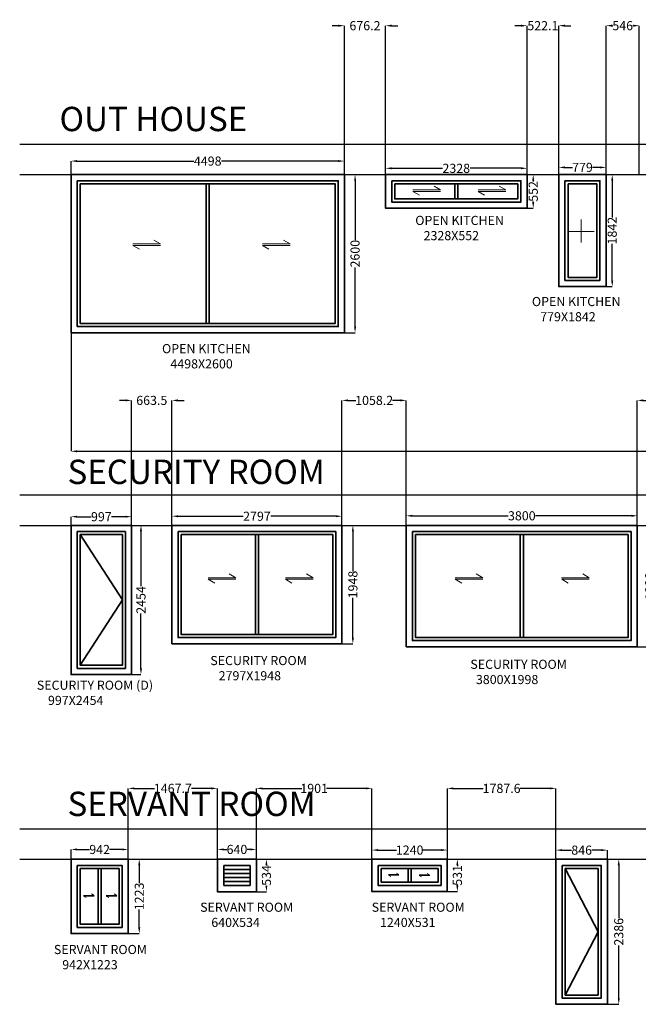
# Model space of a CAD drawing. Units: millimetres. Extents: x 16338 to 57165, y -4429 to 26237.
# Tile 4 of 6: x 18335 to 28512, y 10044 to 26237. Entities that reach past the tile are written whole.
import ezdxf

# ---------------------------------------------------------------- set-up
doc = ezdxf.new("R2010")
doc.units = ezdxf.units.MM
doc.header["$MEASUREMENT"] = 0
for name, color, linetype, lineweight in [('A-ANNO-DIMS', 5, 'Continuous', 18), ('A-ANNO-SYMB', 4, 'Continuous', 18), ('A-ANNO-TEXT', 3, 'Continuous', 18), ('A-ELEV', 8, 'Continuous', 25), ('A-GLAZ', 7, 'Continuous', 35)]:
    doc.layers.add(name, color=color, linetype=linetype, lineweight=lineweight)
doc.styles.get("Standard").update_dxf_attribs({"font": 'arial.ttf'})
doc.dimstyles.get("Standard").update_dxf_attribs({"dimtxt": 150, "dimasz": 100, "dimexe": 0.18, "dimexo": 0.0625, "dimgap": 0.09, "dimtad": 0, "dimdec": 0, "dimzin": 0, "dimdsep": 46, "dimtxsty": 'Standard', "dimcen": 0.09, "dimadec": 0, "dimazin": 0, "dimtfac": 1, "dimtdec": 0, "dimtofl": 0, "dimtmove": 0, "dimatfit": 3, "dimfxl": 1, "dimtolj": 1, "dimtzin": 0, "dimarcsym": 0})

# ---------------------------------------------------------------- blocks, each defined once
blk = doc.blocks.new('*D1')
at = {"layer": 'A-ANNO-DIMS', "color": 0, "lineweight": -2, "transparency": 16777216}
for p, q in [((23677, 23689), (23853, 23689)), ((23852, 23589), (23852, 22614)), ((23852, 21189), (23852, 22164)), ((23677, 21089), (23853, 21089))]:
    blk.add_line(p, q, dxfattribs=at)
at = {"layer": 'A-ANNO-DIMS', "color": 0, "transparency": 16777216}
for points in [[(23836, 23589), (23869, 23589), (23852, 23689)], [(23836, 21189), (23869, 21189), (23852, 21089)]]:
    blk.add_solid(points, dxfattribs=at)
at = {"layer": 'Defpoints', "color": 0, "transparency": 16777216}
for p in [(23677, 23689), (23677, 21089), (23852, 21089)]:
    blk.add_point(p, dxfattribs=at)
at = {"layer": 'A-ANNO-DIMS', "color": 0, "transparency": 16777216, "insert": (23852, 22389), "char_height": 150, "attachment_point": 5, "rotation": 90}
blk.add_mtext('\\A1;2600', dxfattribs=at)
blk = doc.blocks.new('*D2')
at = {"layer": 'A-ANNO-DIMS', "color": 0, "lineweight": -2, "transparency": 16777216}
for p, q in [((24353, 23689), (24353, 23793)), ((24453, 23793), (25292, 23793)), ((26581, 23793), (25743, 23793)), ((26681, 23689), (26681, 23793))]:
    blk.add_line(p, q, dxfattribs=at)
at = {"layer": 'A-ANNO-DIMS', "color": 0, "transparency": 16777216}
for points in [[(24453, 23810), (24453, 23777), (24353, 23793)], [(26581, 23810), (26581, 23777), (26681, 23793)]]:
    blk.add_solid(points, dxfattribs=at)
at = {"layer": 'Defpoints', "color": 0, "transparency": 16777216}
for p in [(24353, 23689), (26681, 23793), (26681, 23689)]:
    blk.add_point(p, dxfattribs=at)
at = {"layer": 'A-ANNO-DIMS', "color": 0, "transparency": 16777216, "insert": (25517, 23793), "char_height": 150, "attachment_point": 5}
blk.add_mtext('\\A1;2328', dxfattribs=at)
blk = doc.blocks.new('*D3')
at = {"layer": 'A-ANNO-DIMS', "color": 0, "lineweight": -2, "transparency": 16777216}
for p, q in [((26681, 23689), (26783, 23689)), ((26783, 23589), (26783, 23578)), ((26783, 23237), (26783, 23248)), ((26681, 23137), (26783, 23137))]:
    blk.add_line(p, q, dxfattribs=at)
at = {"layer": 'A-ANNO-DIMS', "color": 0, "transparency": 16777216}
for points in [[(26766, 23589), (26799, 23589), (26783, 23689)], [(26766, 23237), (26799, 23237), (26783, 23137)]]:
    blk.add_solid(points, dxfattribs=at)
at = {"layer": 'Defpoints', "color": 0, "transparency": 16777216}
for p in [(26681, 23689), (26681, 23137), (26783, 23137)]:
    blk.add_point(p, dxfattribs=at)
at = {"layer": 'A-ANNO-DIMS', "color": 0, "transparency": 16777216, "insert": (26783, 23413), "char_height": 150, "attachment_point": 5, "rotation": 90}
blk.add_mtext('\\A1;552', dxfattribs=at)
blk = doc.blocks.new('*D4')
at = {"layer": 'A-ANNO-DIMS', "color": 0, "lineweight": -2, "transparency": 16777216}
for p, q in [((27203, 23689), (27203, 23808)), ((27303, 23808), (27428, 23808)), ((27882, 23808), (27758, 23808)), ((27982, 23689), (27982, 23808))]:
    blk.add_line(p, q, dxfattribs=at)
at = {"layer": 'A-ANNO-DIMS', "color": 0, "transparency": 16777216}
for points in [[(27303, 23824), (27303, 23791), (27203, 23808)], [(27882, 23824), (27882, 23791), (27982, 23808)]]:
    blk.add_solid(points, dxfattribs=at)
at = {"layer": 'Defpoints', "color": 0, "transparency": 16777216}
for p in [(27982, 23808), (27203, 23689), (27982, 23689)]:
    blk.add_point(p, dxfattribs=at)
at = {"layer": 'A-ANNO-DIMS', "color": 0, "transparency": 16777216, "insert": (27593, 23808), "char_height": 150, "attachment_point": 5}
blk.add_mtext('\\A1;779', dxfattribs=at)
blk = doc.blocks.new('*D5')
at = {"layer": 'A-ANNO-DIMS', "color": 0, "lineweight": -2, "transparency": 16777216}
for p, q in [((27982, 23689), (28083, 23689)), ((28082, 23589), (28082, 22984)), ((28082, 21947), (28082, 22552)), ((27982, 21847), (28083, 21847))]:
    blk.add_line(p, q, dxfattribs=at)
at = {"layer": 'A-ANNO-DIMS', "color": 0, "transparency": 16777216}
for points in [[(28066, 23589), (28099, 23589), (28082, 23689)], [(28066, 21947), (28099, 21947), (28082, 21847)]]:
    blk.add_solid(points, dxfattribs=at)
at = {"layer": 'Defpoints', "color": 0, "transparency": 16777216}
for p in [(27982, 23689), (27982, 21847), (28082, 21847)]:
    blk.add_point(p, dxfattribs=at)
at = {"layer": 'A-ANNO-DIMS', "color": 0, "transparency": 16777216, "insert": (28082, 22768), "char_height": 150, "attachment_point": 5, "rotation": 90}
blk.add_mtext('\\A1;1842', dxfattribs=at)
blk = doc.blocks.new('*D20')
at = {"layer": 'A-ANNO-DIMS', "color": 0, "lineweight": -2, "transparency": 16777216}
for p, q in [((19179, 17921), (19179, 18063)), ((19279, 18063), (19512, 18063)), ((20076, 18063), (19843, 18063)), ((20176, 17921), (20176, 18063))]:
    blk.add_line(p, q, dxfattribs=at)
at = {"layer": 'A-ANNO-DIMS', "color": 0, "transparency": 16777216}
for points in [[(19279, 18080), (19279, 18047), (19179, 18063)], [(20076, 18080), (20076, 18047), (20176, 18063)]]:
    blk.add_solid(points, dxfattribs=at)
at = {"layer": 'Defpoints', "color": 0, "transparency": 16777216}
for p in [(20176, 18063), (19179, 17921), (20176, 17921)]:
    blk.add_point(p, dxfattribs=at)
at = {"layer": 'A-ANNO-DIMS', "color": 0, "transparency": 16777216, "insert": (19678, 18063), "char_height": 150, "attachment_point": 5}
blk.add_mtext('\\A1;997', dxfattribs=at)
blk = doc.blocks.new('*D21')
at = {"layer": 'A-ANNO-DIMS', "color": 0, "lineweight": -2, "transparency": 16777216}
for p, q in [((20176, 17921), (20330, 17921)), ((20330, 17821), (20330, 16919)), ((20330, 15567), (20330, 16469)), ((20176, 15467), (20330, 15467))]:
    blk.add_line(p, q, dxfattribs=at)
at = {"layer": 'A-ANNO-DIMS', "color": 0, "transparency": 16777216}
for points in [[(20313, 17821), (20347, 17821), (20330, 17921)], [(20313, 15567), (20347, 15567), (20330, 15467)]]:
    blk.add_solid(points, dxfattribs=at)
at = {"layer": 'Defpoints', "color": 0, "transparency": 16777216}
for p in [(20176, 17921), (20176, 15467), (20330, 15467)]:
    blk.add_point(p, dxfattribs=at)
at = {"layer": 'A-ANNO-DIMS', "color": 0, "transparency": 16777216, "insert": (20330, 16694), "char_height": 150, "attachment_point": 5, "rotation": 90}
blk.add_mtext('\\A1;2454', dxfattribs=at)
blk = doc.blocks.new('*D22')
at = {"layer": 'A-ANNO-DIMS', "color": 0, "lineweight": -2, "transparency": 16777216}
for p, q in [((20840, 17921), (20840, 18071)), ((20940, 18071), (22013, 18071)), ((23537, 18071), (22464, 18071)), ((23637, 17921), (23637, 18071))]:
    blk.add_line(p, q, dxfattribs=at)
at = {"layer": 'A-ANNO-DIMS', "color": 0, "transparency": 16777216}
for points in [[(20940, 18087), (20940, 18054), (20840, 18071)], [(23537, 18087), (23537, 18054), (23637, 18071)]]:
    blk.add_solid(points, dxfattribs=at)
at = {"layer": 'Defpoints', "color": 0, "transparency": 16777216}
for p in [(23637, 18071), (20840, 17921), (23637, 17921)]:
    blk.add_point(p, dxfattribs=at)
at = {"layer": 'A-ANNO-DIMS', "color": 0, "transparency": 16777216, "insert": (22238, 18071), "char_height": 150, "attachment_point": 5}
blk.add_mtext('\\A1;2797', dxfattribs=at)
blk = doc.blocks.new('*D23')
at = {"layer": 'A-ANNO-DIMS', "color": 0, "lineweight": -2, "transparency": 16777216}
for p, q in [((23637, 17921), (23816, 17921)), ((23816, 17821), (23816, 17164)), ((23816, 16073), (23816, 16730)), ((23637, 15973), (23816, 15973))]:
    blk.add_line(p, q, dxfattribs=at)
at = {"layer": 'A-ANNO-DIMS', "color": 0, "transparency": 16777216}
for points in [[(23799, 17821), (23833, 17821), (23816, 17921)], [(23799, 16073), (23833, 16073), (23816, 15973)]]:
    blk.add_solid(points, dxfattribs=at)
at = {"layer": 'Defpoints', "color": 0, "transparency": 16777216}
for p in [(23637, 17921), (23637, 15973), (23816, 15973)]:
    blk.add_point(p, dxfattribs=at)
at = {"layer": 'A-ANNO-DIMS', "color": 0, "transparency": 16777216, "insert": (23816, 16947), "char_height": 150, "attachment_point": 5, "rotation": 90}
blk.add_mtext('\\A1;1948', dxfattribs=at)
blk = doc.blocks.new('*D24')
at = {"layer": 'A-ANNO-DIMS', "color": 0, "lineweight": -2, "transparency": 16777216}
for p, q in [((24695, 17921), (24695, 18078)), ((24795, 18078), (26371, 18078)), ((28395, 18078), (26819, 18078)), ((28495, 17921), (28495, 18078))]:
    blk.add_line(p, q, dxfattribs=at)
at = {"layer": 'A-ANNO-DIMS', "color": 0, "transparency": 16777216}
for points in [[(24795, 18095), (24795, 18061), (24695, 18078)], [(28395, 18095), (28395, 18061), (28495, 18078)]]:
    blk.add_solid(points, dxfattribs=at)
at = {"layer": 'Defpoints', "color": 0, "transparency": 16777216}
for p in [(28495, 18078), (24695, 17921), (28495, 17921)]:
    blk.add_point(p, dxfattribs=at)
at = {"layer": 'A-ANNO-DIMS', "color": 0, "transparency": 16777216, "insert": (26595, 18078), "char_height": 150, "attachment_point": 5}
blk.add_mtext('\\A1;3800', dxfattribs=at)
blk = doc.blocks.new('*D25')
at = {"layer": 'A-ANNO-DIMS', "color": 0, "lineweight": -2, "transparency": 16777216}
for p, q in [((28495, 17921), (28700, 17921)), ((28700, 17821), (28700, 17139)), ((28700, 16023), (28700, 16705)), ((28495, 15923), (28700, 15923))]:
    blk.add_line(p, q, dxfattribs=at)
at = {"layer": 'A-ANNO-DIMS', "color": 0, "transparency": 16777216}
for points in [[(28683, 17821), (28717, 17821), (28700, 17921)], [(28683, 16023), (28717, 16023), (28700, 15923)]]:
    blk.add_solid(points, dxfattribs=at)
at = {"layer": 'Defpoints', "color": 0, "transparency": 16777216}
for p in [(28495, 17921), (28495, 15923), (28700, 15923)]:
    blk.add_point(p, dxfattribs=at)
at = {"layer": 'A-ANNO-DIMS', "color": 0, "transparency": 16777216, "insert": (28700, 16922), "char_height": 150, "attachment_point": 5, "rotation": 90}
blk.add_mtext('\\A1;1998', dxfattribs=at)
blk = doc.blocks.new('*D40')
at = {"layer": 'A-ANNO-DIMS', "color": 0, "lineweight": -2, "transparency": 16777216}
for p, q in [((19179, 12430), (19179, 12591)), ((19279, 12590), (19485, 12590)), ((20021, 12590), (19815, 12590)), ((20121, 12430), (20121, 12591))]:
    blk.add_line(p, q, dxfattribs=at)
at = {"layer": 'A-ANNO-DIMS', "color": 0, "transparency": 16777216}
for points in [[(19279, 12607), (19279, 12574), (19179, 12590)], [(20021, 12607), (20021, 12574), (20121, 12590)]]:
    blk.add_solid(points, dxfattribs=at)
at = {"layer": 'Defpoints', "color": 0, "transparency": 16777216}
for p in [(20121, 12590), (19179, 12430), (20121, 12430)]:
    blk.add_point(p, dxfattribs=at)
at = {"layer": 'A-ANNO-DIMS', "color": 0, "transparency": 16777216, "insert": (19650, 12590), "char_height": 150, "attachment_point": 5}
blk.add_mtext('\\A1;942', dxfattribs=at)
blk = doc.blocks.new('*D41')
at = {"layer": 'A-ANNO-DIMS', "color": 0, "lineweight": -2, "transparency": 16777216}
for p, q in [((20121, 12430), (20302, 12430)), ((20302, 12330), (20302, 12035)), ((20302, 11307), (20302, 11601)), ((20121, 11207), (20302, 11207))]:
    blk.add_line(p, q, dxfattribs=at)
at = {"layer": 'A-ANNO-DIMS', "color": 0, "transparency": 16777216}
for points in [[(20285, 12330), (20318, 12330), (20302, 12430)], [(20285, 11307), (20318, 11307), (20302, 11207)]]:
    blk.add_solid(points, dxfattribs=at)
at = {"layer": 'Defpoints', "color": 0, "transparency": 16777216}
for p in [(20121, 12430), (20121, 11207), (20302, 11207)]:
    blk.add_point(p, dxfattribs=at)
at = {"layer": 'A-ANNO-DIMS', "color": 0, "transparency": 16777216, "insert": (20302, 11818), "char_height": 150, "attachment_point": 5, "rotation": 90}
blk.add_mtext('\\A1;1223', dxfattribs=at)
blk = doc.blocks.new('*D42')
at = {"layer": 'A-ANNO-DIMS', "color": 0, "lineweight": -2, "transparency": 16777216}
for p, q in [((21589, 12430), (21589, 12591)), ((21689, 12591), (21743, 12591)), ((22129, 12591), (22075, 12591)), ((22229, 12430), (22229, 12591))]:
    blk.add_line(p, q, dxfattribs=at)
at = {"layer": 'A-ANNO-DIMS', "color": 0, "transparency": 16777216}
for points in [[(21689, 12607), (21689, 12574), (21589, 12591)], [(22129, 12607), (22129, 12574), (22229, 12591)]]:
    blk.add_solid(points, dxfattribs=at)
at = {"layer": 'Defpoints', "color": 0, "transparency": 16777216}
for p in [(22229, 12591), (21589, 12430), (22229, 12430)]:
    blk.add_point(p, dxfattribs=at)
at = {"layer": 'A-ANNO-DIMS', "color": 0, "transparency": 16777216, "insert": (21909, 12591), "char_height": 150, "attachment_point": 5}
blk.add_mtext('\\A1;640', dxfattribs=at)
blk = doc.blocks.new('*D43')
at = {"layer": 'A-ANNO-DIMS', "color": 0, "lineweight": -2, "transparency": 16777216}
for p, q in [((22229, 12430), (22394, 12430)), ((22394, 12330), (22394, 12328)), ((22394, 11996), (22394, 11997)), ((22229, 11896), (22394, 11896))]:
    blk.add_line(p, q, dxfattribs=at)
at = {"layer": 'A-ANNO-DIMS', "color": 0, "transparency": 16777216}
for points in [[(22377, 12330), (22410, 12330), (22394, 12430)], [(22377, 11996), (22410, 11996), (22394, 11896)]]:
    blk.add_solid(points, dxfattribs=at)
at = {"layer": 'Defpoints', "color": 0, "transparency": 16777216}
for p in [(22229, 12430), (22229, 11896), (22394, 11896)]:
    blk.add_point(p, dxfattribs=at)
at = {"layer": 'A-ANNO-DIMS', "color": 0, "transparency": 16777216, "insert": (22394, 12163), "char_height": 150, "attachment_point": 5, "rotation": 90}
blk.add_mtext('\\A1;534', dxfattribs=at)
blk = doc.blocks.new('*D44')
at = {"layer": 'A-ANNO-DIMS', "color": 0, "lineweight": -2, "transparency": 16777216}
for p, q in [((24130, 12430), (24130, 12581)), ((24230, 12580), (24533, 12580)), ((25270, 12580), (24966, 12580)), ((25370, 12430), (25370, 12581))]:
    blk.add_line(p, q, dxfattribs=at)
at = {"layer": 'A-ANNO-DIMS', "color": 0, "transparency": 16777216}
for points in [[(24230, 12597), (24230, 12564), (24130, 12580)], [(25270, 12597), (25270, 12564), (25370, 12580)]]:
    blk.add_solid(points, dxfattribs=at)
at = {"layer": 'Defpoints', "color": 0, "transparency": 16777216}
for p in [(25370, 12580), (24130, 12430), (25370, 12430)]:
    blk.add_point(p, dxfattribs=at)
at = {"layer": 'A-ANNO-DIMS', "color": 0, "transparency": 16777216, "insert": (24750, 12580), "char_height": 150, "attachment_point": 5}
blk.add_mtext('\\A1;1240', dxfattribs=at)
blk = doc.blocks.new('*D45')
at = {"layer": 'A-ANNO-DIMS', "color": 0, "lineweight": -2, "transparency": 16777216}
for p, q in [((25370, 12430), (25535, 12430)), ((25535, 12330), (25535, 12315)), ((25535, 11999), (25535, 12013)), ((25370, 11899), (25535, 11899))]:
    blk.add_line(p, q, dxfattribs=at)
at = {"layer": 'A-ANNO-DIMS', "color": 0, "transparency": 16777216}
for points in [[(25518, 12330), (25551, 12330), (25535, 12430)], [(25518, 11999), (25551, 11999), (25535, 11899)]]:
    blk.add_solid(points, dxfattribs=at)
at = {"layer": 'Defpoints', "color": 0, "transparency": 16777216}
for p in [(25370, 12430), (25370, 11899), (25535, 11899)]:
    blk.add_point(p, dxfattribs=at)
at = {"layer": 'A-ANNO-DIMS', "color": 0, "transparency": 16777216, "insert": (25535, 12164), "char_height": 150, "attachment_point": 5, "rotation": 90}
blk.add_mtext('\\A1;531', dxfattribs=at)
blk = doc.blocks.new('*D46')
at = {"layer": 'A-ANNO-DIMS', "color": 0, "lineweight": -2, "transparency": 16777216}
for p, q in [((27157, 12430), (27157, 12580)), ((27257, 12579), (27414, 12579)), ((27903, 12579), (27746, 12579)), ((28003, 12430), (28003, 12580))]:
    blk.add_line(p, q, dxfattribs=at)
at = {"layer": 'A-ANNO-DIMS', "color": 0, "transparency": 16777216}
for points in [[(27257, 12596), (27257, 12563), (27157, 12579)], [(27903, 12596), (27903, 12563), (28003, 12579)]]:
    blk.add_solid(points, dxfattribs=at)
at = {"layer": 'Defpoints', "color": 0, "transparency": 16777216}
for p in [(28003, 12579), (27157, 12430), (28003, 12430)]:
    blk.add_point(p, dxfattribs=at)
at = {"layer": 'A-ANNO-DIMS', "color": 0, "transparency": 16777216, "insert": (27580, 12579), "char_height": 150, "attachment_point": 5}
blk.add_mtext('\\A1;846', dxfattribs=at)
blk = doc.blocks.new('*D47')
at = {"layer": 'A-ANNO-DIMS', "color": 0, "lineweight": -2, "transparency": 16777216}
for p, q in [((28003, 12430), (28190, 12430)), ((28190, 12330), (28190, 11462)), ((28190, 10144), (28190, 11011)), ((28003, 10044), (28190, 10044))]:
    blk.add_line(p, q, dxfattribs=at)
at = {"layer": 'A-ANNO-DIMS', "color": 0, "transparency": 16777216}
for points in [[(28173, 12330), (28207, 12330), (28190, 12430)], [(28173, 10144), (28207, 10144), (28190, 10044)]]:
    blk.add_solid(points, dxfattribs=at)
at = {"layer": 'Defpoints', "color": 0, "transparency": 16777216}
for p in [(28003, 12430), (28003, 10044), (28190, 10044)]:
    blk.add_point(p, dxfattribs=at)
at = {"layer": 'A-ANNO-DIMS', "color": 0, "transparency": 16777216, "insert": (28190, 11237), "char_height": 150, "attachment_point": 5, "rotation": 90}
blk.add_mtext('\\A1;2386', dxfattribs=at)
blk = doc.blocks.new('*D77')
at = {"layer": 'A-ANNO-DIMS', "color": 0, "lineweight": -2, "transparency": 16777216}
for p, q in [((19179, 23689), (19179, 23912)), ((19279, 23912), (21201, 23912)), ((23577, 23912), (21655, 23912)), ((23677, 23689), (23677, 23912))]:
    blk.add_line(p, q, dxfattribs=at)
at = {"layer": 'A-ANNO-DIMS', "color": 0, "transparency": 16777216}
for points in [[(19279, 23929), (19279, 23896), (19179, 23912)], [(23577, 23929), (23577, 23896), (23677, 23912)]]:
    blk.add_solid(points, dxfattribs=at)
at = {"layer": 'Defpoints', "color": 0, "transparency": 16777216}
for p in [(23677, 23912), (19179, 23689), (23677, 23689)]:
    blk.add_point(p, dxfattribs=at)
at = {"layer": 'A-ANNO-DIMS', "color": 0, "transparency": 16777216, "insert": (21428, 23912), "char_height": 150, "attachment_point": 5}
blk.add_mtext('\\A1;4498', dxfattribs=at)
blk = doc.blocks.new('SLIDE-ARROW-L')
for p, q in [((454, 0), (347, 62)), ((0, 0), (454, 0))]:
    blk.add_line(p, q)
blk = doc.blocks.new('SLIDE-ARROW-S')
for p, q in [((173, 0), (132, 24)), ((0, 0), (173, 0))]:
    blk.add_line(p, q)
blk = doc.blocks.new('*D82')
at = {"layer": 'A-ANNO-DIMS', "color": 0, "lineweight": -2, "transparency": 16777216}
for p, q in [((23577, 26139), (23477, 26139)), ((23677, 23689), (23677, 26139)), ((24353, 23689), (24353, 26139)), ((24453, 26139), (24553, 26139))]:
    blk.add_line(p, q, dxfattribs=at)
at = {"layer": 'A-ANNO-DIMS', "color": 0, "transparency": 16777216}
for points in [[(23577, 26156), (23577, 26122), (23677, 26139)], [(24453, 26156), (24453, 26122), (24353, 26139)]]:
    blk.add_solid(points, dxfattribs=at)
at = {"layer": 'Defpoints', "color": 0, "transparency": 16777216}
for p in [(24353, 26139), (23677, 23689), (24353, 23689)]:
    blk.add_point(p, dxfattribs=at)
at = {"layer": 'A-ANNO-DIMS', "color": 0, "transparency": 16777216, "insert": (24015, 26139), "char_height": 150, "attachment_point": 5}
blk.add_mtext('\\A1;676.2', dxfattribs=at)
blk = doc.blocks.new('*D83')
at = {"layer": 'A-ANNO-DIMS', "color": 0, "lineweight": -2, "transparency": 16777216}
for p, q in [((26581, 26139), (26481, 26139)), ((26681, 23689), (26681, 26139)), ((27203, 23689), (27203, 26139)), ((27303, 26139), (27403, 26139))]:
    blk.add_line(p, q, dxfattribs=at)
at = {"layer": 'A-ANNO-DIMS', "color": 0, "transparency": 16777216}
for points in [[(26581, 26156), (26581, 26122), (26681, 26139)], [(27303, 26156), (27303, 26122), (27203, 26139)]]:
    blk.add_solid(points, dxfattribs=at)
at = {"layer": 'Defpoints', "color": 0, "transparency": 16777216}
for p in [(27203, 26139), (26681, 23689), (27203, 23689)]:
    blk.add_point(p, dxfattribs=at)
at = {"layer": 'A-ANNO-DIMS', "color": 0, "transparency": 16777216, "insert": (26942, 26139), "char_height": 150, "attachment_point": 5}
blk.add_mtext('\\A1;522.1', dxfattribs=at)
blk = doc.blocks.new('*D84')
at = {"layer": 'A-ANNO-DIMS', "color": 0, "lineweight": -2, "transparency": 16777216}
for p, q in [((27982, 23689), (27982, 26139)), ((28082, 26139), (28090, 26139)), ((28428, 26139), (28421, 26139)), ((28528, 23689), (28528, 26139))]:
    blk.add_line(p, q, dxfattribs=at)
at = {"layer": 'A-ANNO-DIMS', "color": 0, "transparency": 16777216}
for points in [[(28082, 26156), (28082, 26122), (27982, 26139)], [(28428, 26156), (28428, 26122), (28528, 26139)]]:
    blk.add_solid(points, dxfattribs=at)
at = {"layer": 'Defpoints', "color": 0, "transparency": 16777216}
for p in [(28528, 26139), (27982, 23689), (28528, 23689)]:
    blk.add_point(p, dxfattribs=at)
at = {"layer": 'A-ANNO-DIMS', "color": 0, "transparency": 16777216, "insert": (28255, 26139), "char_height": 150, "attachment_point": 5}
blk.add_mtext('\\A1;546', dxfattribs=at)
blk = doc.blocks.new('*D91')
at = {"layer": 'A-ANNO-DIMS', "color": 0, "lineweight": -2, "transparency": 16777216}
for p, q in [((19179, 21089), (19179, 19139)), ((54667, 21100), (54667, 19139)), ((19279, 19139), (36641, 19139)), ((54567, 19139), (37205, 19139))]:
    blk.add_line(p, q, dxfattribs=at)
at = {"layer": 'A-ANNO-DIMS', "color": 0, "transparency": 16777216}
for points in [[(19279, 19156), (19279, 19122), (19179, 19139)], [(54567, 19156), (54567, 19122), (54667, 19139)]]:
    blk.add_solid(points, dxfattribs=at)
at = {"layer": 'Defpoints', "color": 0, "transparency": 16777216}
for p in [(19179, 21089), (54667, 21100), (54667, 19139)]:
    blk.add_point(p, dxfattribs=at)
at = {"layer": 'A-ANNO-DIMS', "color": 0, "transparency": 16777216, "insert": (36923, 19139), "char_height": 150, "attachment_point": 5}
blk.add_mtext('\\A1;35487', dxfattribs=at)
blk = doc.blocks.new('*D95')
at = {"layer": 'A-ANNO-DIMS', "color": 0, "lineweight": -2, "transparency": 16777216}
for p, q in [((20076, 19976), (19976, 19976)), ((20176, 17921), (20176, 19976)), ((20840, 17921), (20840, 19976)), ((20940, 19976), (21040, 19976))]:
    blk.add_line(p, q, dxfattribs=at)
at = {"layer": 'A-ANNO-DIMS', "color": 0, "transparency": 16777216}
for points in [[(20076, 19993), (20076, 19959), (20176, 19976)], [(20940, 19993), (20940, 19959), (20840, 19976)]]:
    blk.add_solid(points, dxfattribs=at)
at = {"layer": 'Defpoints', "color": 0, "transparency": 16777216}
for p in [(20840, 19976), (20176, 17921), (20840, 17921)]:
    blk.add_point(p, dxfattribs=at)
at = {"layer": 'A-ANNO-DIMS', "color": 0, "transparency": 16777216, "insert": (20508, 19976), "char_height": 150, "attachment_point": 5}
blk.add_mtext('\\A1;663.5', dxfattribs=at)
blk = doc.blocks.new('*D96')
at = {"layer": 'A-ANNO-DIMS', "color": 0, "lineweight": -2, "transparency": 16777216}
for p, q in [((23637, 17921), (23637, 19976)), ((23737, 19976), (23862, 19976)), ((24595, 19976), (24469, 19976)), ((24695, 17921), (24695, 19976))]:
    blk.add_line(p, q, dxfattribs=at)
at = {"layer": 'A-ANNO-DIMS', "color": 0, "transparency": 16777216}
for points in [[(23737, 19993), (23737, 19959), (23637, 19976)], [(24595, 19993), (24595, 19959), (24695, 19976)]]:
    blk.add_solid(points, dxfattribs=at)
at = {"layer": 'Defpoints', "color": 0, "transparency": 16777216}
for p in [(24695, 19976), (23637, 17921), (24695, 17921)]:
    blk.add_point(p, dxfattribs=at)
at = {"layer": 'A-ANNO-DIMS', "color": 0, "transparency": 16777216, "insert": (24166, 19976), "char_height": 150, "attachment_point": 5}
blk.add_mtext('\\A1;1058.2', dxfattribs=at)
blk = doc.blocks.new('*D97')
at = {"layer": 'A-ANNO-DIMS', "color": 0, "lineweight": -2, "transparency": 16777216}
for p, q in [((28495, 17921), (28495, 19976)), ((28595, 19976), (28736, 19976)), ((29210, 19976), (29069, 19976)), ((29310, 17921), (29310, 19976))]:
    blk.add_line(p, q, dxfattribs=at)
at = {"layer": 'A-ANNO-DIMS', "color": 0, "transparency": 16777216}
for points in [[(28595, 19993), (28595, 19959), (28495, 19976)], [(29210, 19993), (29210, 19959), (29310, 19976)]]:
    blk.add_solid(points, dxfattribs=at)
at = {"layer": 'Defpoints', "color": 0, "transparency": 16777216}
for p in [(29310, 19976), (28495, 17921), (29310, 17921)]:
    blk.add_point(p, dxfattribs=at)
at = {"layer": 'A-ANNO-DIMS', "color": 0, "transparency": 16777216, "insert": (28902, 19976), "char_height": 150, "attachment_point": 5}
blk.add_mtext('\\A1;815', dxfattribs=at)
blk = doc.blocks.new('*D104')
at = {"layer": 'A-ANNO-DIMS', "color": 0, "lineweight": -2, "transparency": 16777216}
for p, q in [((20121, 12430), (20121, 13595)), ((20221, 13595), (20551, 13595)), ((21489, 13595), (21159, 13595)), ((21589, 12430), (21589, 13595))]:
    blk.add_line(p, q, dxfattribs=at)
at = {"layer": 'A-ANNO-DIMS', "color": 0, "transparency": 16777216}
for points in [[(20221, 13611), (20221, 13578), (20121, 13595)], [(21489, 13611), (21489, 13578), (21589, 13595)]]:
    blk.add_solid(points, dxfattribs=at)
at = {"layer": 'Defpoints', "color": 0, "transparency": 16777216}
for p in [(21589, 13595), (20121, 12430), (21589, 12430)]:
    blk.add_point(p, dxfattribs=at)
at = {"layer": 'A-ANNO-DIMS', "color": 0, "transparency": 16777216, "insert": (20855, 13595), "char_height": 150, "attachment_point": 5}
blk.add_mtext('\\A1;1467.7', dxfattribs=at)
blk = doc.blocks.new('*D105')
at = {"layer": 'A-ANNO-DIMS', "color": 0, "lineweight": -2, "transparency": 16777216}
for p, q in [((22229, 12430), (22229, 13595)), ((22329, 13595), (22977, 13595)), ((24030, 13595), (23382, 13595)), ((24130, 12430), (24130, 13595))]:
    blk.add_line(p, q, dxfattribs=at)
at = {"layer": 'A-ANNO-DIMS', "color": 0, "transparency": 16777216}
for points in [[(22329, 13611), (22329, 13578), (22229, 13595)], [(24030, 13611), (24030, 13578), (24130, 13595)]]:
    blk.add_solid(points, dxfattribs=at)
at = {"layer": 'Defpoints', "color": 0, "transparency": 16777216}
for p in [(24130, 13595), (22229, 12430), (24130, 12430)]:
    blk.add_point(p, dxfattribs=at)
at = {"layer": 'A-ANNO-DIMS', "color": 0, "transparency": 16777216, "insert": (23179, 13595), "char_height": 150, "attachment_point": 5}
blk.add_mtext('\\A1;1901', dxfattribs=at)
blk = doc.blocks.new('*D106')
at = {"layer": 'A-ANNO-DIMS', "color": 0, "lineweight": -2, "transparency": 16777216}
for p, q in [((25370, 12430), (25370, 13595)), ((25470, 13595), (25959, 13595)), ((27057, 13595), (26568, 13595)), ((27157, 12430), (27157, 13595))]:
    blk.add_line(p, q, dxfattribs=at)
at = {"layer": 'A-ANNO-DIMS', "color": 0, "transparency": 16777216}
for points in [[(25470, 13611), (25470, 13578), (25370, 13595)], [(27057, 13611), (27057, 13578), (27157, 13595)]]:
    blk.add_solid(points, dxfattribs=at)
at = {"layer": 'Defpoints', "color": 0, "transparency": 16777216}
for p in [(27157, 13595), (25370, 12430), (27157, 12430)]:
    blk.add_point(p, dxfattribs=at)
at = {"layer": 'A-ANNO-DIMS', "color": 0, "transparency": 16777216, "insert": (26263, 13595), "char_height": 150, "attachment_point": 5}
blk.add_mtext('\\A1;1787.6', dxfattribs=at)

msp = doc.modelspace()

# ---------------------------------------------------------------- linework, layer by layer
at = {"layer": 'A-ANNO-DIMS'}
for p in [(21690.43, 12261.83), (21690.43, 12195.67), (21690.43, 12129.51), (21690.43, 12063.35)]:
    msp.add_point(p, dxfattribs=at)
at = {"layer": 'A-ANNO-SYMB'}
for p, q in [((27569.64, 22571.93), (27569.64, 22950.15)), ((27355.23, 22753.02), (27784.05, 22753.02))]:
    msp.add_line(p, q, dxfattribs=at)
at = {"layer": 'A-ELEV'}
for p, q in [((18334.8, 24189.02), (57164.77, 24189.02)), ((18334.8, 23689.02), (57154.46, 23689.02)), ((18334.8, 18421.15), (49111.23, 18421.15)), ((18334.8, 17921.15), (49122.07, 17921.15)), ((18334.8, 12929.59), (29250.98, 12929.59)), ((18334.8, 12429.59), (29267.6, 12429.59))]:
    msp.add_line(p, q, dxfattribs=at)
at = {"layer": 'A-GLAZ'}
for p, q in [((21402.77, 23536.62), (21402.77, 21241.42)), ((21453.57, 23536.62), (21453.57, 21241.42)), ((25491.92, 23289.42), (25491.92, 23536.62)), ((25542.72, 23289.42), (25542.72, 23536.62)), ((19331.57, 17768.75), (20023.77, 16694.15)), ((22212.8, 16125.55), (22212.8, 17768.75)), ((22263.6, 16125.55), (22263.6, 17768.75)), ((26569.52, 16075.55), (26569.52, 17768.75)), ((26620.32, 16075.55), (26620.32, 17768.75)), ((20023.77, 16694.15), (19331.57, 15619.55)), ((21690.43, 12327.99), (22127.23, 12327.99)), ((21690.43, 11997.19), (21690.43, 12327.99)), ((22127.23, 12327.99), (22127.23, 11997.19)), ((19624.77, 11358.99), (19624.77, 12277.19)), ((19675.57, 11358.99), (19675.57, 12277.19)), ((21690.43, 12261.83), (22127.23, 12261.83)), ((21690.43, 12195.67), (22127.23, 12195.67)), ((24724.31, 12277.19), (24724.31, 12050.99)), ((24775.11, 12277.19), (24775.11, 12050.99)), ((27309.66, 12277.19), (27850.86, 11236.59)), ((21690.43, 12129.51), (22127.23, 12129.51)), ((21690.43, 12063.35), (22127.23, 12063.35)), ((22127.23, 11997.19), (21690.43, 11997.19)), ((27850.86, 11236.59), (27309.66, 10195.99))]:
    msp.add_line(p, q, dxfattribs=at)
for points in [[(19179.17, 23689.02), (23677.17, 23689.02), (23677.17, 21089.02), (19179.17, 21089.02)], [(24353.32, 23689.02), (26681.32, 23689.02), (26681.32, 23137.02), (24353.32, 23137.02)], [(27203.39, 23689.02), (27982.39, 23689.02), (27982.39, 21847.02), (27203.39, 21847.02)], [(19280.77, 23587.42), (23575.57, 23587.42), (23575.57, 21190.62), (19280.77, 21190.62)], [(19331.57, 23536.62), (23524.77, 23536.62), (23524.77, 21241.42), (19331.57, 21241.42)], [(24454.92, 23587.42), (26579.72, 23587.42), (26579.72, 23238.62), (24454.92, 23238.62)], [(24505.72, 23536.62), (26528.92, 23536.62), (26528.92, 23289.42), (24505.72, 23289.42)], [(27304.99, 23587.42), (27880.79, 23587.42), (27880.79, 21948.62), (27304.99, 21948.62)], [(27355.79, 23536.62), (27829.99, 23536.62), (27829.99, 21999.42), (27355.79, 21999.42)], [(19179.17, 17921.15), (20176.17, 17921.15), (20176.17, 15467.15), (19179.17, 15467.15)], [(19280.77, 17819.55), (20074.57, 17819.55), (20074.57, 15568.75), (19280.77, 15568.75)], [(20839.7, 17921.15), (23636.7, 17921.15), (23636.7, 15973.15), (20839.7, 15973.15)], [(20941.3, 17819.55), (23535.1, 17819.55), (23535.1, 16074.75), (20941.3, 16074.75)], [(24694.92, 17921.15), (28494.92, 17921.15), (28494.92, 15923.15), (24694.92, 15923.15)], [(24796.52, 17819.55), (28393.32, 17819.55), (28393.32, 16024.75), (24796.52, 16024.75)], [(19331.57, 17768.75), (20023.77, 17768.75), (20023.77, 15619.55), (19331.57, 15619.55)], [(20992.1, 17768.75), (23484.3, 17768.75), (23484.3, 16125.55), (20992.1, 16125.55)], [(24847.32, 17768.75), (28342.52, 17768.75), (28342.52, 16075.55), (24847.32, 16075.55)], [(19179.17, 12429.59), (20121.17, 12429.59), (20121.17, 11206.59), (19179.17, 11206.59)], [(19280.77, 12327.99), (20019.57, 12327.99), (20019.57, 11308.19), (19280.77, 11308.19)], [(21588.83, 12429.59), (22228.83, 12429.59), (22228.83, 11895.59), (21588.83, 11895.59)], [(24129.71, 12429.59), (25369.71, 12429.59), (25369.71, 11898.59), (24129.71, 11898.59)], [(24231.31, 12327.99), (25268.11, 12327.99), (25268.11, 12000.19), (24231.31, 12000.19)], [(27157.26, 12429.59), (28003.26, 12429.59), (28003.26, 10043.59), (27157.26, 10043.59)], [(27258.86, 12327.99), (27901.66, 12327.99), (27901.66, 10145.19), (27258.86, 10145.19)], [(19331.57, 12277.19), (19968.77, 12277.19), (19968.77, 11358.99), (19331.57, 11358.99)], [(24282.11, 12277.19), (25217.31, 12277.19), (25217.31, 12050.99), (24282.11, 12050.99)], [(27309.66, 12277.19), (27850.86, 12277.19), (27850.86, 10195.99), (27309.66, 10195.99)]]:
    msp.add_lwpolyline(points, close=True, dxfattribs=at)

# ---------------------------------------------------------------- block references
at = {"layer": 'A-ANNO-SYMB'}
for name, p in [('SLIDE-ARROW-L', (24803.61, 23437.6)), ('SLIDE-ARROW-L', (25876.66, 23437.6)), ('SLIDE-ARROW-L', (20196.4, 22550.65)), ('SLIDE-ARROW-L', (22328.89, 22550.65)), ('SLIDE-ARROW-L', (21435.71, 17059.37)), ('SLIDE-ARROW-L', (22707.34, 17059.37)), ('SLIDE-ARROW-L', (25499.28, 17059.37)), ('SLIDE-ARROW-L', (27250.75, 17059.37)), ('SLIDE-ARROW-S', (24401.03, 12177.91)), ('SLIDE-ARROW-S', (24906.02, 12173.61)), ('SLIDE-ARROW-S', (19385.93, 11834.04)), ('SLIDE-ARROW-S', (19757.42, 11834.04))]:
    msp.add_blockref(name, p, dxfattribs=at)
at = {"layer": 'A-ANNO-SYMB', "rotation": 180}
for name, p in [('SLIDE-ARROW-L', (25257.81, 23412.95)), ('SLIDE-ARROW-L', (26330.86, 23412.95)), ('SLIDE-ARROW-L', (20650.6, 22525.99)), ('SLIDE-ARROW-L', (22783.09, 22525.99)), ('SLIDE-ARROW-L', (21889.91, 17034.72)), ('SLIDE-ARROW-L', (23161.54, 17034.72)), ('SLIDE-ARROW-L', (25953.48, 17034.72)), ('SLIDE-ARROW-L', (27704.95, 17034.72)), ('SLIDE-ARROW-S', (24574.34, 12168.51)), ('SLIDE-ARROW-S', (25079.33, 12164.21)), ('SLIDE-ARROW-S', (19559.24, 11824.63)), ('SLIDE-ARROW-S', (19930.73, 11824.63))]:
    msp.add_blockref(name, p, dxfattribs=at)

# ---------------------------------------------------------------- texts
at = {"layer": 'A-ANNO-TEXT', "attachment_point": 1}
for s, insert, char_height in [('OUT HOUSE', (18989.57, 24804.45), 400), ('OPEN KITCHEN\\P   2328X552', (24842.11, 23011.26), 150), ('OPEN KITCHEN\\P   779X1842', (26760.84, 21676.95), 150), ('OPEN KITCHEN\\P   4498X2600', (20676.57, 20902.28), 150), ('SECURITY ROOM', (19121.7, 19001.06), 400), ('SECURITY ROOM \\P   2797X1948', (21470.64, 15772.3), 150), ('SECURITY ROOM \\P  3800X1998', (25748.68, 15710.34), 150), ('SECURITY ROOM (D)\\P    997X2454', (18616.82, 15367.06), 150), ('SERVANT ROOM', (19121.7, 13540.41), 400), ('SERVANT ROOM \\P    640X534', (21303.7, 11715.49), 150), ('SERVANT ROOM \\P   1240X531', (24125.44, 11715.49), 150), ('SERVANT ROOM\\P   942X1223', (18897.65, 11020.01), 150)]:
    msp.add_mtext_dynamic_manual_height_columns(s, width=7094.9176, gutter_width=1, heights=[0], dxfattribs=dict(at, insert=insert, char_height=char_height))

# ---------------------------------------------------------------- dimensions: what is measured, and where the dimension line sits
at = {"layer": 'A-ANNO-DIMS'}
for base, p1, p2, override, picture, middle in [((24353.3248, 26139.016), (23677.169, 23689.016), (24353.3248, 23689.016), {"dimdec": 1, "dimlfac": 1, "dimrnd": 0, "dimzin": 0, "dimdsep": 46, "dimlunit": 2}, '*D82', (24015.2469, 26139.016)), ((27203.39, 26139.02), (26681.32, 23689.02), (27203.39, 23689.02), {"dimdec": 1, "dimlfac": 1, "dimrnd": 0, "dimzin": 0, "dimdsep": 46, "dimlunit": 2}, '*D83', (26942.36, 26139.02)), ((28528.37, 26139.02), (27982.39, 23689.02), (28528.37, 23689.02), {"dimdec": 0, "dimlfac": 1, "dimrnd": 0, "dimzin": 0, "dimdsep": 46, "dimlunit": 2}, '*D84', (28255.38, 26139.02)), ((23677.17, 23912.32), (19179.17, 23689.02), (23677.17, 23689.02), {"dimclrd": 0, "dimclre": 0, "dimclrt": 0}, '*D77', (21428.17, 23912.32)), ((26681.32, 23793.27), (24353.32, 23689.02), (26681.32, 23689.02), {"dimclrd": 0, "dimclre": 0, "dimclrt": 0}, '*D2', (25517.32, 23793.27)), ((27982.39, 23807.59), (27203.39, 23689.02), (27982.39, 23689.02), {"dimclrd": 0, "dimclre": 0, "dimclrt": 0}, '*D4', (27592.89, 23807.59)), ((54666.53, 19139.02), (19179.17, 21089.02), (54666.53, 21100.02), {"dimdec": 0, "dimlfac": 1, "dimrnd": 0, "dimzin": 0, "dimdsep": 46, "dimlunit": 2}, '*D91', (36922.85, 19139.02)), ((20839.7, 19976.15), (20176.17, 17921.15), (20839.7, 17921.15), {"dimdec": 1, "dimlfac": 1, "dimrnd": 0, "dimzin": 0, "dimdsep": 46, "dimlunit": 2}, '*D95', (20507.93, 19976.15)), ((24694.92, 19976.15), (23636.7, 17921.15), (24694.92, 17921.15), {"dimdec": 1, "dimlfac": 1, "dimrnd": 0, "dimzin": 0, "dimdsep": 46, "dimlunit": 2}, '*D96', (24165.81, 19976.15)), ((29309.84, 19976.15), (28494.92, 17921.15), (29309.84, 17921.15), {"dimdec": 0, "dimlfac": 1, "dimrnd": 0, "dimzin": 0, "dimdsep": 46, "dimlunit": 2}, '*D97', (28902.38, 19976.15)), ((20176.17, 18063.19), (19179.17, 17921.15), (20176.17, 17921.15), {"dimclrd": 0, "dimclre": 0, "dimclrt": 0}, '*D20', (19677.67, 18063.19)), ((23636.7, 18070.5), (20839.7, 17921.15), (23636.7, 17921.15), {"dimclrd": 0, "dimclre": 0, "dimclrt": 0}, '*D22', (22238.2, 18070.5)), ((28494.92, 18077.84), (24694.92, 17921.15), (28494.92, 17921.15), {"dimclrd": 0, "dimclre": 0, "dimclrt": 0}, '*D24', (26594.92, 18077.84)), ((21588.83, 13594.59), (20121.17, 12429.59), (21588.83, 12429.59), {"dimdec": 1, "dimlfac": 1, "dimrnd": 0, "dimzin": 0, "dimdsep": 46, "dimlunit": 2}, '*D104', (20855, 13594.59)), ((24129.71, 13594.59), (22228.83, 12429.59), (24129.71, 12429.59), {"dimdec": 0, "dimlfac": 1, "dimrnd": 0, "dimzin": 0, "dimdsep": 46, "dimlunit": 2}, '*D105', (23179.27, 13594.59)), ((27157.2607, 13594.5883), (25369.7066, 12429.5883), (27157.2607, 12429.5883), {"dimdec": 1, "dimlfac": 1, "dimrnd": 0, "dimzin": 0, "dimdsep": 46, "dimlunit": 2}, '*D106', (26263.4837, 13594.5883)), ((20121.17, 12590.38), (19179.17, 12429.59), (20121.17, 12429.59), {"dimclrd": 0, "dimclre": 0, "dimclrt": 0}, '*D40', (19650.17, 12590.38)), ((22228.83, 12590.82), (21588.83, 12429.59), (22228.83, 12429.59), {"dimclrd": 0, "dimclre": 0, "dimclrt": 0}, '*D42', (21908.83, 12590.82)), ((25369.71, 12580.45), (24129.71, 12429.59), (25369.71, 12429.59), {"dimclrd": 0, "dimclre": 0, "dimclrt": 0}, '*D44', (24749.71, 12580.45)), ((28003.26, 12579.48), (27157.26, 12429.59), (28003.26, 12429.59), {"dimclrd": 0, "dimclre": 0, "dimclrt": 0}, '*D46', (27580.26, 12579.48))]:
    dim = msp.add_linear_dim(base=base, p1=p1, p2=p2, dimstyle='Standard', override=override, dxfattribs=at)
    dim.commit()
    dim.dimension.update_dxf_attribs({"geometry": picture, "text_midpoint": middle})
for base, p1, p2, picture, middle in [((23852.4, 21089.02), (23677.17, 23689.02), (23677.17, 21089.02), '*D1', (23852.4, 22389.02)), ((26782.83, 23137.02), (26681.32, 23689.02), (26681.32, 23137.02), '*D3', (26782.83, 23413.02)), ((28082.42, 21847.02), (27982.39, 23689.02), (27982.39, 21847.02), '*D5', (28082.42, 22768.02)), ((20330.01, 15467.15), (20176.17, 17921.15), (20176.17, 15467.15), '*D21', (20330.01, 16694.15)), ((23816.11, 15973.15), (23636.7, 17921.15), (23636.7, 15973.15), '*D23', (23816.11, 16947.15)), ((28699.97, 15923.15), (28494.92, 17921.15), (28494.92, 15923.15), '*D25', (28699.97, 16922.15)), ((20301.59, 11206.59), (20121.17, 12429.59), (20121.17, 11206.59), '*D41', (20301.59, 11818.09)), ((22393.59, 11895.59), (22228.83, 12429.59), (22228.83, 11895.59), '*D43', (22393.59, 12162.59)), ((25534.55, 11898.59), (25369.71, 12429.59), (25369.71, 11898.59), '*D45', (25534.55, 12164.09)), ((28190.14, 10043.59), (28003.26, 12429.59), (28003.26, 10043.59), '*D47', (28190.14, 11236.59))]:
    dim = msp.add_linear_dim(base=base, p1=p1, p2=p2, angle=90, dimstyle='Standard', override={"dimclrd": 0, "dimclre": 0, "dimclrt": 0}, dxfattribs=at)
    dim.commit()
    dim.dimension.update_dxf_attribs({"geometry": picture, "text_midpoint": middle})

doc.saveas('drawing.dxf')
